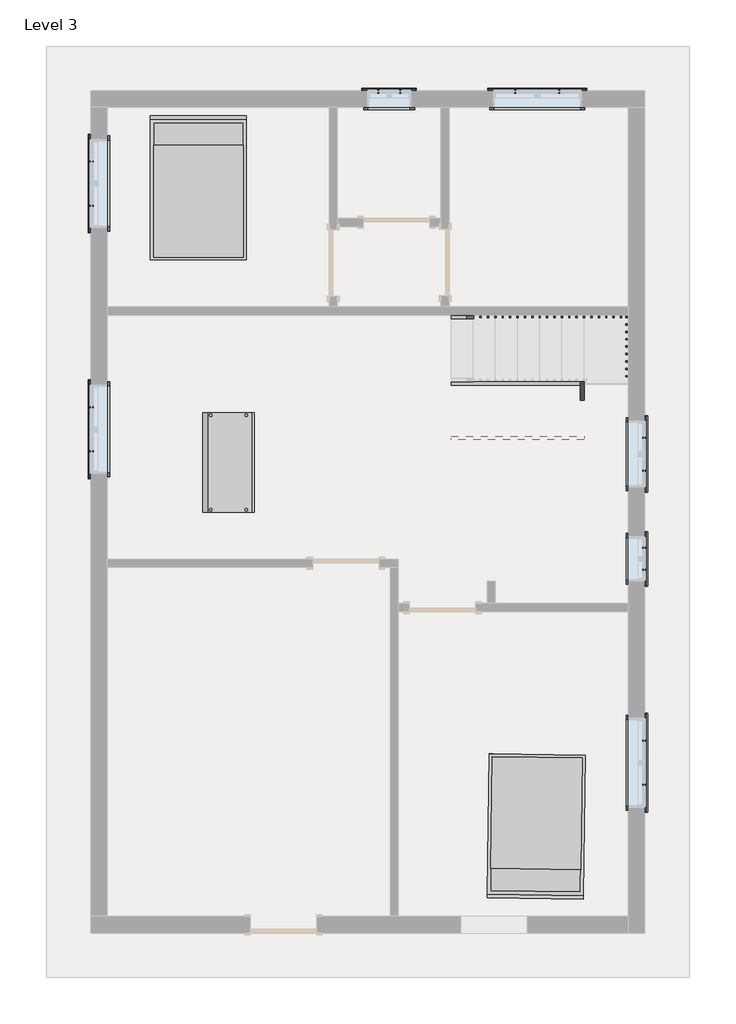
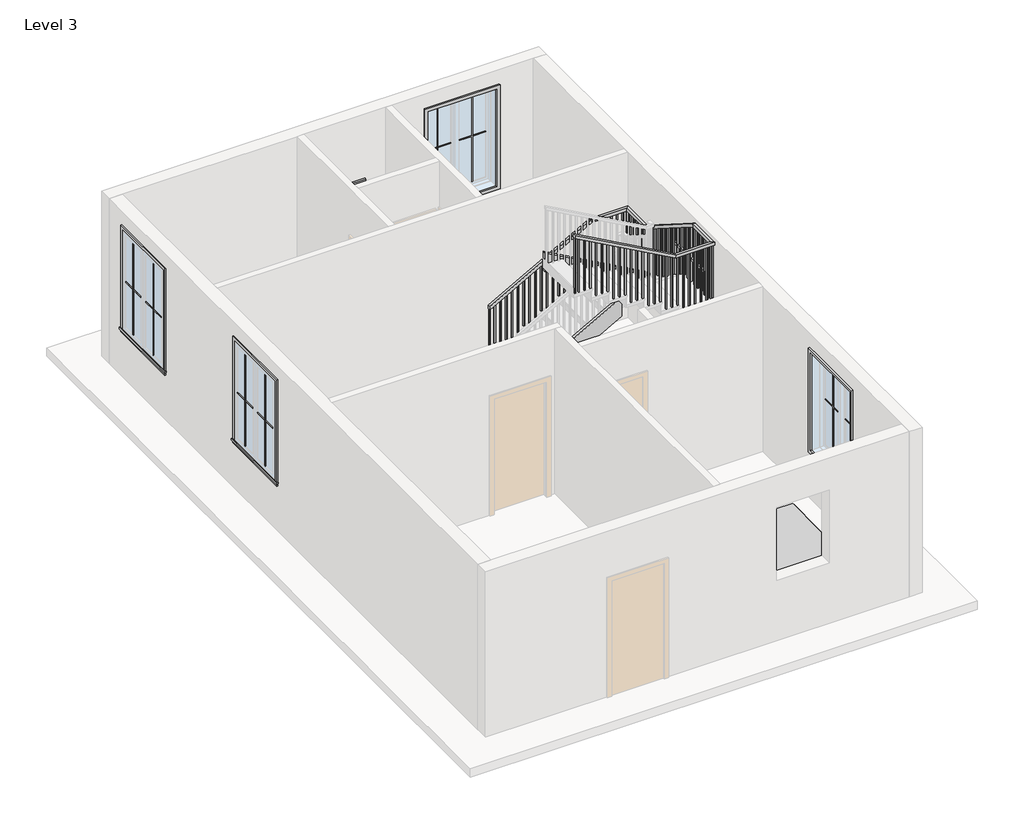
# One storey, part 2 of 2: 29 proxies, 3 members, 2 furniture elements, 1 railing.
"""IFC4 building model written with IfcOpenShell, lengths in millimetres."""

from ifc_helpers import new_model, si_unit, frame, origin, place, context, project, spatial, polyline, outline, extrude, faceted_brep, transform, mapped, element, save
from components import modern_coffee_table_17989_modern_coffee_table_17989_d3a860c8, muntin_pattern_2x2_muntin_pattern_2x2_2b4d9f72, muntin_pattern_2x2_muntin_pattern_2x2_ef995ed3, muntin_pattern_2x2_muntin_pattern_2x2_53152e2c, muntin_pattern_2x2_muntin_pattern_2x2_e8f3e573, muntin_pattern_2x2_muntin_pattern_2x2_9b64c8d5, muntin_pattern_2x2_muntin_pattern_2x2_d319fd2e, trim_window_exterior_flat_with_sill_b7e4d11c, trim_window_exterior_flat_with_sill_a665a915, trim_window_exterior_flat_with_sill_66148908, trim_window_interior_flat_picture_frame_936b8d2a, trim_window_interior_flat_picture_frame_d485c387, trim_window_interior_flat_picture_frame_d5b7f3a4, bed_17739_bed_17739_15c61121

model = new_model("IFC4")

# Units and contexts
model_context = context("Model", 3, world=origin())
ifc_project = project(units=[si_unit("LENGTHUNIT", "METRE", prefix="MILLI")], contexts=[model_context])

# Site, building, storey
site = spatial("IfcSite", under=ifc_project)
building = spatial("IfcBuilding", under=site)
storey = spatial("IfcBuildingStorey", under=building, Name="Level 3", Elevation=6096.0)

# Proxies
placement = place(None, origin())
modern_coffee_table_17989_modern_coffee_table_17989_shape = modern_coffee_table_17989_modern_coffee_table_17989_d3a860c8(model_context)
element("IfcBuildingElementProxy", 1, Name="Modern_Coffee_Table_17989 : Modern_Coffee_Table_17989", ObjectType="Modern_Coffee_Table_17989 : Modern_Coffee_Table_17989", at=placement, inside=storey, context=model_context, shape_type="MappedRepresentation", body=[
    mapped(modern_coffee_table_17989_modern_coffee_table_17989_shape, transform((3060.7, 9172.1823212, 6096.0), x_axis=(0.0, 1.0, 0.0), y_axis=(-1.0, 0.0, 0.0), z_axis=(0.0, 0.0, 1.0))),
])
muntin_pattern_2x2_muntin_pattern_2x2_shape = muntin_pattern_2x2_muntin_pattern_2x2_2b4d9f72(model_context)
element("IfcBuildingElementProxy", 2, Name="Muntin Pattern_2x2 : Muntin Pattern_2x2", ObjectType="Muntin Pattern_2x2 : Muntin Pattern_2x2", at=placement, inside=storey, context=model_context, shape_type="MappedRepresentation", body=[
    mapped(muntin_pattern_2x2_muntin_pattern_2x2_shape, transform((1533.525, 12477.4069306, 7080.25), x_axis=(0.0, 1.0, 0.0), y_axis=(-1.0, 0.0, 0.0), z_axis=(0.0, 0.0, 1.0))),
])
element("IfcBuildingElementProxy", 3, Name="Muntin Pattern_2x2 : Muntin Pattern_2x2", ObjectType="Muntin Pattern_2x2 : Muntin Pattern_2x2", at=placement, inside=storey, context=model_context, shape_type="MappedRepresentation", body=[
    mapped(muntin_pattern_2x2_muntin_pattern_2x2_shape, transform((7361.2375, 14045.8073212, 7080.25), x_axis=(1.0, 0.0, 0.0), y_axis=(0.0, 1.0, 0.0), z_axis=(0.0, 0.0, 1.0))),
])
element("IfcBuildingElementProxy", 4, Name="Muntin Pattern_2x2 : Muntin Pattern_2x2", ObjectType="Muntin Pattern_2x2 : Muntin Pattern_2x2", at=placement, inside=storey, context=model_context, shape_type="MappedRepresentation", body=[
    mapped(muntin_pattern_2x2_muntin_pattern_2x2_shape, transform((9134.475, 5119.2948212, 7080.25), x_axis=(0.0, -1.0, 0.0), y_axis=(1.0, 0.0, 0.0), z_axis=(0.0, 0.0, 1.0))),
])
element("IfcBuildingElementProxy", 5, Name="Muntin Pattern_2x2 : Muntin Pattern_2x2", ObjectType="Muntin Pattern_2x2 : Muntin Pattern_2x2", at=placement, inside=storey, context=model_context, shape_type="MappedRepresentation", body=[
    mapped(muntin_pattern_2x2_muntin_pattern_2x2_shape, transform((1533.525, 9097.5698212, 7080.25), x_axis=(0.0, 1.0, 0.0), y_axis=(-1.0, 0.0, 0.0), z_axis=(0.0, 0.0, 1.0))),
])
muntin_pattern_2x2_muntin_pattern_2x2_2_shape = muntin_pattern_2x2_muntin_pattern_2x2_ef995ed3(model_context)
element("IfcBuildingElementProxy", 6, Name="Muntin Pattern_2x2 : Muntin Pattern_2x2", ObjectType="Muntin Pattern_2x2 : Muntin Pattern_2x2", at=placement, inside=storey, context=model_context, shape_type="MappedRepresentation", body=[
    mapped(muntin_pattern_2x2_muntin_pattern_2x2_2_shape, transform((1533.525, 13083.8319306, 7080.25), x_axis=(0.0, -1.0, 0.0), y_axis=(1.0, 0.0, 0.0), z_axis=(0.0, 0.0, 1.0))),
])
element("IfcBuildingElementProxy", 7, Name="Muntin Pattern_2x2 : Muntin Pattern_2x2", ObjectType="Muntin Pattern_2x2 : Muntin Pattern_2x2", at=placement, inside=storey, context=model_context, shape_type="MappedRepresentation", body=[
    mapped(muntin_pattern_2x2_muntin_pattern_2x2_2_shape, transform((7967.6625, 14045.8073212, 7080.25), x_axis=(-1.0, 0.0, 0.0), y_axis=(0.0, -1.0, 0.0), z_axis=(0.0, 0.0, 1.0))),
])
element("IfcBuildingElementProxy", 8, Name="Muntin Pattern_2x2 : Muntin Pattern_2x2", ObjectType="Muntin Pattern_2x2 : Muntin Pattern_2x2", at=placement, inside=storey, context=model_context, shape_type="MappedRepresentation", body=[
    mapped(muntin_pattern_2x2_muntin_pattern_2x2_2_shape, transform((9134.475, 4512.8698212, 7080.25), x_axis=(0.0, 1.0, 0.0), y_axis=(-1.0, 0.0, 0.0), z_axis=(0.0, 0.0, 1.0))),
])
element("IfcBuildingElementProxy", 9, Name="Muntin Pattern_2x2 : Muntin Pattern_2x2", ObjectType="Muntin Pattern_2x2 : Muntin Pattern_2x2", at=placement, inside=storey, context=model_context, shape_type="MappedRepresentation", body=[
    mapped(muntin_pattern_2x2_muntin_pattern_2x2_2_shape, transform((1533.525, 9703.9948212, 7080.25), x_axis=(0.0, -1.0, 0.0), y_axis=(1.0, 0.0, 0.0), z_axis=(0.0, 0.0, 1.0))),
])
muntin_pattern_2x2_muntin_pattern_2x2_3_shape = muntin_pattern_2x2_muntin_pattern_2x2_53152e2c(model_context)
element("IfcBuildingElementProxy", 10, Name="Muntin Pattern_2x2 : Muntin Pattern_2x2", ObjectType="Muntin Pattern_2x2 : Muntin Pattern_2x2", at=placement, inside=storey, context=model_context, shape_type="MappedRepresentation", body=[
    mapped(muntin_pattern_2x2_muntin_pattern_2x2_3_shape, transform((9134.475, 7771.2135712, 7080.25), x_axis=(0.0, -1.0, 0.0), y_axis=(1.0, 0.0, 0.0), z_axis=(0.0, 0.0, 1.0))),
])
element("IfcBuildingElementProxy", 11, Name="Muntin Pattern_2x2 : Muntin Pattern_2x2", ObjectType="Muntin Pattern_2x2 : Muntin Pattern_2x2", at=placement, inside=storey, context=model_context, shape_type="MappedRepresentation", body=[
    mapped(muntin_pattern_2x2_muntin_pattern_2x2_3_shape, transform((5475.2875, 14045.8073212, 7080.25), x_axis=(1.0, 0.0, 0.0), y_axis=(0.0, 1.0, 0.0), z_axis=(0.0, 0.0, 1.0))),
])
muntin_pattern_2x2_muntin_pattern_2x2_4_shape = muntin_pattern_2x2_muntin_pattern_2x2_e8f3e573(model_context)
element("IfcBuildingElementProxy", 12, Name="Muntin Pattern_2x2 : Muntin Pattern_2x2", ObjectType="Muntin Pattern_2x2 : Muntin Pattern_2x2", at=placement, inside=storey, context=model_context, shape_type="MappedRepresentation", body=[
    mapped(muntin_pattern_2x2_muntin_pattern_2x2_4_shape, transform((9134.475, 7469.5885712, 7080.25), x_axis=(0.0, 1.0, 0.0), y_axis=(-1.0, 0.0, 0.0), z_axis=(0.0, 0.0, 1.0))),
])
element("IfcBuildingElementProxy", 13, Name="Muntin Pattern_2x2 : Muntin Pattern_2x2", ObjectType="Muntin Pattern_2x2 : Muntin Pattern_2x2", at=placement, inside=storey, context=model_context, shape_type="MappedRepresentation", body=[
    mapped(muntin_pattern_2x2_muntin_pattern_2x2_4_shape, transform((5776.9125, 14045.8073212, 7080.25), x_axis=(-1.0, 0.0, 0.0), y_axis=(0.0, -1.0, 0.0), z_axis=(0.0, 0.0, 1.0))),
])
muntin_pattern_2x2_muntin_pattern_2x2_5_shape = muntin_pattern_2x2_muntin_pattern_2x2_9b64c8d5(model_context)
element("IfcBuildingElementProxy", 14, Name="Muntin Pattern_2x2 : Muntin Pattern_2x2", ObjectType="Muntin Pattern_2x2 : Muntin Pattern_2x2", at=placement, inside=storey, context=model_context, shape_type="MappedRepresentation", body=[
    mapped(muntin_pattern_2x2_muntin_pattern_2x2_5_shape, transform((9134.475, 9287.1024384, 7080.25), x_axis=(0.0, -1.0, 0.0), y_axis=(1.0, 0.0, 0.0), z_axis=(0.0, 0.0, 1.0))),
])
muntin_pattern_2x2_muntin_pattern_2x2_6_shape = muntin_pattern_2x2_muntin_pattern_2x2_d319fd2e(model_context)
element("IfcBuildingElementProxy", 15, Name="Muntin Pattern_2x2 : Muntin Pattern_2x2", ObjectType="Muntin Pattern_2x2 : Muntin Pattern_2x2", at=placement, inside=storey, context=model_context, shape_type="MappedRepresentation", body=[
    mapped(muntin_pattern_2x2_muntin_pattern_2x2_6_shape, transform((9134.475, 8833.0774384, 7080.25), x_axis=(0.0, 1.0, 0.0), y_axis=(-1.0, 0.0, 0.0), z_axis=(0.0, 0.0, 1.0))),
])
trim_window_exterior_flat_with_sill_shape = trim_window_exterior_flat_with_sill_b7e4d11c(model_context)
element("IfcBuildingElementProxy", 16, Name="Trim-Window-Exterior-Flat : with Sill", ObjectType="Trim-Window-Exterior-Flat : with Sill", at=placement, inside=storey, context=model_context, shape_type="MappedRepresentation", body=[
    mapped(trim_window_exterior_flat_with_sill_shape, transform((1524.0, 12780.6194306, 8839.2), x_axis=(0.0, -1.0, 0.0), y_axis=(0.0, 0.0, 1.0), z_axis=(-1.0, 0.0, 0.0))),
])
element("IfcBuildingElementProxy", 17, Name="Trim-Window-Exterior-Flat : with Sill", ObjectType="Trim-Window-Exterior-Flat : with Sill", at=placement, inside=storey, context=model_context, shape_type="MappedRepresentation", body=[
    mapped(trim_window_exterior_flat_with_sill_shape, transform((7664.45, 14055.3323212, 8839.2), x_axis=(-1.0, 0.0, 0.0), y_axis=(0.0, 0.0, 1.0), z_axis=(0.0, 1.0, 0.0))),
])
element("IfcBuildingElementProxy", 18, Name="Trim-Window-Exterior-Flat : with Sill", ObjectType="Trim-Window-Exterior-Flat : with Sill", at=placement, inside=storey, context=model_context, shape_type="MappedRepresentation", body=[
    mapped(trim_window_exterior_flat_with_sill_shape, transform((9144.0, 4816.0823212, 8839.2), x_axis=(0.0, 1.0, 0.0), y_axis=(0.0, 0.0, 1.0), z_axis=(1.0, 0.0, 0.0))),
])
element("IfcBuildingElementProxy", 19, Name="Trim-Window-Exterior-Flat : with Sill", ObjectType="Trim-Window-Exterior-Flat : with Sill", at=placement, inside=storey, context=model_context, shape_type="MappedRepresentation", body=[
    mapped(trim_window_exterior_flat_with_sill_shape, transform((1524.0, 9400.7823212, 8839.2), x_axis=(0.0, -1.0, 0.0), y_axis=(0.0, 0.0, 1.0), z_axis=(-1.0, 0.0, 0.0))),
])
trim_window_exterior_flat_with_sill_2_shape = trim_window_exterior_flat_with_sill_a665a915(model_context)
element("IfcBuildingElementProxy", 20, Name="Trim-Window-Exterior-Flat : with Sill", ObjectType="Trim-Window-Exterior-Flat : with Sill", at=placement, inside=storey, context=model_context, shape_type="MappedRepresentation", body=[
    mapped(trim_window_exterior_flat_with_sill_2_shape, transform((9144.0, 7620.4010712, 7924.8), x_axis=(0.0, 1.0, 0.0), y_axis=(0.0, 0.0, 1.0), z_axis=(1.0, 0.0, 0.0))),
])
element("IfcBuildingElementProxy", 21, Name="Trim-Window-Exterior-Flat : with Sill", ObjectType="Trim-Window-Exterior-Flat : with Sill", at=placement, inside=storey, context=model_context, shape_type="MappedRepresentation", body=[
    mapped(trim_window_exterior_flat_with_sill_2_shape, transform((5626.1, 14055.3323212, 7924.8), x_axis=(-1.0, 0.0, 0.0), y_axis=(0.0, 0.0, 1.0), z_axis=(0.0, 1.0, 0.0))),
])
trim_window_exterior_flat_with_sill_3_shape = trim_window_exterior_flat_with_sill_66148908(model_context)
element("IfcBuildingElementProxy", 22, Name="Trim-Window-Exterior-Flat : with Sill", ObjectType="Trim-Window-Exterior-Flat : with Sill", at=placement, inside=storey, context=model_context, shape_type="MappedRepresentation", body=[
    mapped(trim_window_exterior_flat_with_sill_3_shape, transform((9144.0, 9060.0899384, 8356.6), x_axis=(0.0, 1.0, 0.0), y_axis=(0.0, 0.0, 1.0), z_axis=(1.0, 0.0, 0.0))),
])
trim_window_interior_flat_picture_frame_shape = trim_window_interior_flat_picture_frame_936b8d2a(model_context)
element("IfcBuildingElementProxy", 23, Name="Trim-Window-Interior-Flat : Picture Frame", ObjectType="Trim-Window-Interior-Flat : Picture Frame", at=placement, inside=storey, context=model_context, shape_type="MappedRepresentation", body=[
    mapped(trim_window_interior_flat_picture_frame_shape, transform((1752.6, 12780.6194306, 8839.2), x_axis=(0.0, 1.0, 0.0), y_axis=(0.0, 0.0, 1.0), z_axis=(1.0, 0.0, 0.0))),
])
element("IfcBuildingElementProxy", 24, Name="Trim-Window-Interior-Flat : Picture Frame", ObjectType="Trim-Window-Interior-Flat : Picture Frame", at=placement, inside=storey, context=model_context, shape_type="MappedRepresentation", body=[
    mapped(trim_window_interior_flat_picture_frame_shape, transform((7664.45, 13826.7323212, 8839.2), x_axis=(1.0, 0.0, 0.0), y_axis=(0.0, 0.0, 1.0), z_axis=(0.0, -1.0, 0.0))),
])
element("IfcBuildingElementProxy", 25, Name="Trim-Window-Interior-Flat : Picture Frame", ObjectType="Trim-Window-Interior-Flat : Picture Frame", at=placement, inside=storey, context=model_context, shape_type="MappedRepresentation", body=[
    mapped(trim_window_interior_flat_picture_frame_shape, transform((8915.4, 4816.0823212, 8839.2), x_axis=(0.0, -1.0, 0.0), y_axis=(0.0, 0.0, 1.0), z_axis=(-1.0, 0.0, 0.0))),
])
element("IfcBuildingElementProxy", 26, Name="Trim-Window-Interior-Flat : Picture Frame", ObjectType="Trim-Window-Interior-Flat : Picture Frame", at=placement, inside=storey, context=model_context, shape_type="MappedRepresentation", body=[
    mapped(trim_window_interior_flat_picture_frame_shape, transform((1752.6, 9400.7823212, 8839.2), x_axis=(0.0, 1.0, 0.0), y_axis=(0.0, 0.0, 1.0), z_axis=(1.0, 0.0, 0.0))),
])
trim_window_interior_flat_picture_frame_2_shape = trim_window_interior_flat_picture_frame_d485c387(model_context)
element("IfcBuildingElementProxy", 27, Name="Trim-Window-Interior-Flat : Picture Frame", ObjectType="Trim-Window-Interior-Flat : Picture Frame", at=placement, inside=storey, context=model_context, shape_type="MappedRepresentation", body=[
    mapped(trim_window_interior_flat_picture_frame_2_shape, transform((8915.4, 7620.4010712, 7924.8), x_axis=(0.0, -1.0, 0.0), y_axis=(0.0, 0.0, 1.0), z_axis=(-1.0, 0.0, 0.0))),
])
element("IfcBuildingElementProxy", 28, Name="Trim-Window-Interior-Flat : Picture Frame", ObjectType="Trim-Window-Interior-Flat : Picture Frame", at=placement, inside=storey, context=model_context, shape_type="MappedRepresentation", body=[
    mapped(trim_window_interior_flat_picture_frame_2_shape, transform((5626.1, 13826.7323212, 7924.8), x_axis=(1.0, 0.0, 0.0), y_axis=(0.0, 0.0, 1.0), z_axis=(0.0, -1.0, 0.0))),
])
trim_window_interior_flat_picture_frame_3_shape = trim_window_interior_flat_picture_frame_d5b7f3a4(model_context)
element("IfcBuildingElementProxy", 29, Name="Trim-Window-Interior-Flat : Picture Frame", ObjectType="Trim-Window-Interior-Flat : Picture Frame", at=placement, inside=storey, context=model_context, shape_type="MappedRepresentation", body=[
    mapped(trim_window_interior_flat_picture_frame_3_shape, transform((8915.4, 9060.0899384, 8356.6), x_axis=(0.0, -1.0, 0.0), y_axis=(0.0, 0.0, 1.0), z_axis=(-1.0, 0.0, 0.0))),
])

# Furniture
bed_17739_bed_17739_shape = bed_17739_bed_17739_15c61121(model_context)
element("IfcFurniture", 30, ObjectType="Bed_17739 : Bed_17739", at=placement, inside=storey, context=model_context, shape_type="MappedRepresentation", body=[
    mapped(bed_17739_bed_17739_shape, transform((3003.55, 12696.4323212, 6096.0), x_axis=(1.0, 0.0, 0.0), y_axis=(0.0, 1.0, 0.0), z_axis=(0.0, 0.0, 1.0))),
])
element("IfcFurniture", 31, ObjectType="Bed_17739 : Bed_17739", at=placement, inside=storey, context=model_context, shape_type="MappedRepresentation", body=[
    mapped(bed_17739_bed_17739_shape, transform((7650.1504891, 3963.5673274, 6096.0), x_axis=(-0.9999063358908578, 0.013686469424921632, 0.0), y_axis=(-0.013686469424921632, -0.9999063358908578, 0.0), z_axis=(0.0, 0.0, 1.0))),
])

# Members
element("IfcMember", 32, ObjectType="Stringer - 2\" Width", at=placement, inside=storey, context=model_context, shape_type="SweptSolid", body=[
    extrude(outline(polyline([(6303.5983948, 6477.0), (6096.0, 6477.0), (6096.0, 6730.9445028), (6942.6974984, 8255.0), (7291.3761726, 8255.0), (6303.5983948, 6477.0)])), frame((0.0, 10004.0323212, 0.0), z_axis=(0.0, 1.0, 0.0), x_axis=(0.0, 0.0, 1.0)), (0.0, 0.0, 1.0), 50.8),
])
element("IfcMember", 33, ObjectType="Stringer - 2\" Width", at=placement, inside=storey, context=model_context, shape_type="SweptSolid", body=[
    extrude(outline(polyline([(10054.8323212, 7496.2030053), (10054.8323212, 7135.1566026), (9305.5323212, 7610.9026344), (9305.5323212, 7971.949037), (10054.8323212, 7496.2030053)])), frame((8255.0, 0.0, 0.0), z_axis=(1.0, 0.0, 0.0), x_axis=(0.0, 1.0, 0.0)), (0.0, 0.0, 1.0), 50.8),
])
element("IfcMember", 34, ObjectType="Stringer - 2\" Width", at=placement, inside=storey, context=model_context, shape_type="SweptSolid", body=[
    extrude(outline(polyline([(7817.5863873, 8305.8), (8166.2650614, 8305.8), (9182.2650614, 6477.0), (8833.5863873, 6477.0), (7817.5863873, 8305.8)])), frame((0.0, 9254.7323212, 0.0), z_axis=(0.0, 1.0, 0.0), x_axis=(0.0, 0.0, 1.0)), (0.0, 0.0, 1.0), 50.8),
])

# Railing
element("IfcRailing", 35, ObjectType="Handrail - Rectangular", at=placement, inside=storey, context=model_context, shape_type="SolidModel", body=[
    faceted_brep([(6477.0, 10969.2323212, 7179.7333333), (6477.0, 10969.2323212, 7121.620221), (6477.0, 10918.4323212, 7121.620221), (6477.0, 10918.4323212, 7179.7333333), (8242.3, 10969.2323212, 8160.4555556), (8255.4636022, 10969.2323212, 8109.6555556), (8255.4636022, 10918.4323212, 8109.6555556), (8242.3, 10918.4323212, 8160.4555556), (8915.4, 10969.2323212, 8160.4555556), (8915.4, 10969.2323212, 8109.6555556), (8864.6, 10918.4323212, 8109.6555556), (8864.6, 10918.4323212, 8160.4555556), (8915.4, 10377.0948212, 8160.4555556), (8915.4, 10362.3301405, 8109.6555556), (8864.6, 10362.3301405, 8109.6555556), (8864.6, 10377.0948212, 8160.4555556), (8915.4, 8932.4698212, 9077.6777778), (8915.4, 8917.7051405, 9026.8777778), (8864.6, 8917.7051405, 9026.8777778), (8864.6, 8932.4698212, 9077.6777778), (8915.4, 8340.3323212, 9077.6777778), (8915.4, 8340.3323212, 9026.8777778), (8864.6, 8391.1323212, 9026.8777778), (8864.6, 8391.1323212, 9077.6777778), (8242.3, 8340.3323212, 9077.6777778), (8229.1363978, 8340.3323212, 9026.8777778), (8229.1363978, 8391.1323212, 9026.8777778), (8242.3, 8391.1323212, 9077.6777778), (6477.0, 8340.3323212, 10058.4), (6477.0, 8391.1323212, 10058.4), (6477.0, 8391.1323212, 10000.2868876), (6477.0, 8340.3323212, 10000.2868876)], [[[0, 1, 2, 3]], [[1, 0, 4, 5]], [[2, 1, 5, 6]], [[3, 2, 6, 7]], [[0, 3, 7, 4]], [[5, 4, 8, 9]], [[6, 5, 9, 10]], [[7, 6, 10, 11]], [[4, 7, 11, 8]], [[9, 8, 12, 13]], [[10, 9, 13, 14]], [[11, 10, 14, 15]], [[8, 11, 15, 12]], [[13, 12, 16, 17]], [[14, 13, 17, 18]], [[15, 14, 18, 19]], [[12, 15, 19, 16]], [[17, 16, 20, 21]], [[18, 17, 21, 22]], [[19, 18, 22, 23]], [[16, 19, 23, 20]], [[21, 20, 24, 25]], [[22, 21, 25, 26]], [[23, 22, 26, 27]], [[20, 23, 27, 24]], [[28, 29, 30, 31]], [[25, 24, 28, 31]], [[26, 25, 31, 30]], [[27, 26, 30, 29]], [[24, 27, 29, 28]]]),
    extrude(outline(polyline([(9963.245221, 6543.675), (8974.6666667, 6543.675), (8974.6666667, 6562.725), (9952.6618876, 6562.725), (9963.245221, 6543.675)])), frame((0.0, 8356.2073212, 0.0), z_axis=(0.0, 1.0, 0.0), x_axis=(0.0, 0.0, 1.0)), (0.0, 0.0, 1.0), 19.05),
    extrude(outline(polyline([(9906.8007765, 6645.275), (8974.6666667, 6645.275), (8974.6666667, 6664.325), (9896.2174432, 6664.325), (9906.8007765, 6645.275)])), frame((0.0, 8356.2073212, 0.0), z_axis=(0.0, 1.0, 0.0), x_axis=(0.0, 0.0, 1.0)), (0.0, 0.0, 1.0), 19.05),
    extrude(outline(polyline([(9850.3563321, 6746.875), (8974.6666667, 6746.875), (8974.6666667, 6765.925), (9839.7729988, 6765.925), (9850.3563321, 6746.875)])), frame((0.0, 8356.2073212, 0.0), z_axis=(0.0, 1.0, 0.0), x_axis=(0.0, 0.0, 1.0)), (0.0, 0.0, 1.0), 19.05),
    extrude(outline(polyline([(9793.9118876, 6848.475), (8805.3333333, 6848.475), (8805.3333333, 6867.525), (9783.3285543, 6867.525), (9793.9118876, 6848.475)])), frame((0.0, 8356.2073212, 0.0), z_axis=(0.0, 1.0, 0.0), x_axis=(0.0, 0.0, 1.0)), (0.0, 0.0, 1.0), 19.05),
    extrude(outline(polyline([(9737.4674432, 6950.075), (8805.3333333, 6950.075), (8805.3333333, 6969.125), (9726.8841099, 6969.125), (9737.4674432, 6950.075)])), frame((0.0, 8356.2073212, 0.0), z_axis=(0.0, 1.0, 0.0), x_axis=(0.0, 0.0, 1.0)), (0.0, 0.0, 1.0), 19.05),
    extrude(outline(polyline([(9681.0229988, 7051.675), (8805.3333333, 7051.675), (8805.3333333, 7070.725), (9670.4396654, 7070.725), (9681.0229988, 7051.675)])), frame((0.0, 8356.2073212, 0.0), z_axis=(0.0, 1.0, 0.0), x_axis=(0.0, 0.0, 1.0)), (0.0, 0.0, 1.0), 19.05),
    extrude(outline(polyline([(9624.5785543, 7153.275), (8636.0, 7153.275), (8636.0, 7172.325), (9613.995221, 7172.325), (9624.5785543, 7153.275)])), frame((0.0, 8356.2073212, 0.0), z_axis=(0.0, 1.0, 0.0), x_axis=(0.0, 0.0, 1.0)), (0.0, 0.0, 1.0), 19.05),
    extrude(outline(polyline([(9568.1341099, 7254.875), (8636.0, 7254.875), (8636.0, 7273.925), (9557.5507765, 7273.925), (9568.1341099, 7254.875)])), frame((0.0, 8356.2073212, 0.0), z_axis=(0.0, 1.0, 0.0), x_axis=(0.0, 0.0, 1.0)), (0.0, 0.0, 1.0), 19.05),
    extrude(outline(polyline([(9511.6896654, 7356.475), (8636.0, 7356.475), (8636.0, 7375.525), (9501.1063321, 7375.525), (9511.6896654, 7356.475)])), frame((0.0, 8356.2073212, 0.0), z_axis=(0.0, 1.0, 0.0), x_axis=(0.0, 0.0, 1.0)), (0.0, 0.0, 1.0), 19.05),
    extrude(outline(polyline([(9455.245221, 7458.075), (8466.6666667, 7458.075), (8466.6666667, 7477.125), (9444.6618876, 7477.125), (9455.245221, 7458.075)])), frame((0.0, 8356.2073212, 0.0), z_axis=(0.0, 1.0, 0.0), x_axis=(0.0, 0.0, 1.0)), (0.0, 0.0, 1.0), 19.05),
    extrude(outline(polyline([(9398.8007765, 7559.675), (8466.6666667, 7559.675), (8466.6666667, 7578.725), (9388.2174432, 7578.725), (9398.8007765, 7559.675)])), frame((0.0, 8356.2073212, 0.0), z_axis=(0.0, 1.0, 0.0), x_axis=(0.0, 0.0, 1.0)), (0.0, 0.0, 1.0), 19.05),
    extrude(outline(polyline([(9342.3563321, 7661.275), (8466.6666667, 7661.275), (8466.6666667, 7680.325), (9331.7729988, 7680.325), (9342.3563321, 7661.275)])), frame((0.0, 8356.2073212, 0.0), z_axis=(0.0, 1.0, 0.0), x_axis=(0.0, 0.0, 1.0)), (0.0, 0.0, 1.0), 19.05),
    extrude(outline(polyline([(9285.9118876, 7762.875), (8297.3333333, 7762.875), (8297.3333333, 7781.925), (9275.3285543, 7781.925), (9285.9118876, 7762.875)])), frame((0.0, 8356.2073212, 0.0), z_axis=(0.0, 1.0, 0.0), x_axis=(0.0, 0.0, 1.0)), (0.0, 0.0, 1.0), 19.05),
    extrude(outline(polyline([(9229.4674432, 7864.475), (8297.3333333, 7864.475), (8297.3333333, 7883.525), (9218.8841099, 7883.525), (9229.4674432, 7864.475)])), frame((0.0, 8356.2073212, 0.0), z_axis=(0.0, 1.0, 0.0), x_axis=(0.0, 0.0, 1.0)), (0.0, 0.0, 1.0), 19.05),
    extrude(outline(polyline([(9173.0229988, 7966.075), (8297.3333333, 7966.075), (8297.3333333, 7985.125), (9162.4396654, 7985.125), (9173.0229988, 7966.075)])), frame((0.0, 8356.2073212, 0.0), z_axis=(0.0, 1.0, 0.0), x_axis=(0.0, 0.0, 1.0)), (0.0, 0.0, 1.0), 19.05),
    extrude(outline(polyline([(9116.5785543, 8067.675), (8128.0, 8067.675), (8128.0, 8086.725), (9105.995221, 8086.725), (9116.5785543, 8067.675)])), frame((0.0, 8356.2073212, 0.0), z_axis=(0.0, 1.0, 0.0), x_axis=(0.0, 0.0, 1.0)), (0.0, 0.0, 1.0), 19.05),
    extrude(outline(polyline([(9060.1341099, 8169.275), (8128.0, 8169.275), (8128.0, 8188.325), (9049.5507765, 8188.325), (9060.1341099, 8169.275)])), frame((0.0, 8356.2073212, 0.0), z_axis=(0.0, 1.0, 0.0), x_axis=(0.0, 0.0, 1.0)), (0.0, 0.0, 1.0), 19.05),
    extrude(outline(polyline([(8289.925, 8356.2073212), (8270.875, 8356.2073212), (8270.875, 8375.2573212), (8289.925, 8375.2573212), (8289.925, 8356.2073212)])), frame((0.0, 0.0, 8128.0), z_axis=(0.0, 0.0, 1.0), x_axis=(1.0, 0.0, 0.0)), (0.0, 0.0, 1.0), 898.8777778),
    extrude(outline(polyline([(8391.525, 8356.2073212), (8372.475, 8356.2073212), (8372.475, 8375.2573212), (8391.525, 8375.2573212), (8391.525, 8356.2073212)])), frame((0.0, 0.0, 7958.6666667), z_axis=(0.0, 0.0, 1.0), x_axis=(1.0, 0.0, 0.0)), (0.0, 0.0, 1.0), 1068.2111111),
    extrude(outline(polyline([(8493.125, 8356.2073212), (8474.075, 8356.2073212), (8474.075, 8375.2573212), (8493.125, 8375.2573212), (8493.125, 8356.2073212)])), frame((0.0, 0.0, 7958.6666667), z_axis=(0.0, 0.0, 1.0), x_axis=(1.0, 0.0, 0.0)), (0.0, 0.0, 1.0), 1068.2111111),
    extrude(outline(polyline([(8594.725, 8356.2073212), (8575.675, 8356.2073212), (8575.675, 8375.2573212), (8594.725, 8375.2573212), (8594.725, 8356.2073212)])), frame((0.0, 0.0, 7958.6666667), z_axis=(0.0, 0.0, 1.0), x_axis=(1.0, 0.0, 0.0)), (0.0, 0.0, 1.0), 1068.2111111),
    extrude(outline(polyline([(8696.325, 8356.2073212), (8677.275, 8356.2073212), (8677.275, 8375.2573212), (8696.325, 8375.2573212), (8696.325, 8356.2073212)])), frame((0.0, 0.0, 7958.6666667), z_axis=(0.0, 0.0, 1.0), x_axis=(1.0, 0.0, 0.0)), (0.0, 0.0, 1.0), 1068.2111111),
    extrude(outline(polyline([(8797.925, 8356.2073212), (8778.875, 8356.2073212), (8778.875, 8375.2573212), (8797.925, 8375.2573212), (8797.925, 8356.2073212)])), frame((0.0, 0.0, 7958.6666667), z_axis=(0.0, 0.0, 1.0), x_axis=(1.0, 0.0, 0.0)), (0.0, 0.0, 1.0), 1068.2111111),
    extrude(outline(polyline([(8899.525, 8413.3573212), (8899.525, 8394.3073212), (8880.475, 8394.3073212), (8880.475, 8413.3573212), (8899.525, 8413.3573212)])), frame((0.0, 0.0, 7958.6666667), z_axis=(0.0, 0.0, 1.0), x_axis=(1.0, 0.0, 0.0)), (0.0, 0.0, 1.0), 1068.2111111),
    extrude(outline(polyline([(8899.525, 8514.9573212), (8899.525, 8495.9073212), (8880.475, 8495.9073212), (8880.475, 8514.9573212), (8899.525, 8514.9573212)])), frame((0.0, 0.0, 7958.6666667), z_axis=(0.0, 0.0, 1.0), x_axis=(1.0, 0.0, 0.0)), (0.0, 0.0, 1.0), 1068.2111111),
    extrude(outline(polyline([(8899.525, 8616.5573212), (8899.525, 8597.5073212), (8880.475, 8597.5073212), (8880.475, 8616.5573212), (8899.525, 8616.5573212)])), frame((0.0, 0.0, 7958.6666667), z_axis=(0.0, 0.0, 1.0), x_axis=(1.0, 0.0, 0.0)), (0.0, 0.0, 1.0), 1068.2111111),
    extrude(outline(polyline([(8899.525, 8718.1573212), (8899.525, 8699.1073212), (8880.475, 8699.1073212), (8880.475, 8718.1573212), (8899.525, 8718.1573212)])), frame((0.0, 0.0, 7958.6666667), z_axis=(0.0, 0.0, 1.0), x_axis=(1.0, 0.0, 0.0)), (0.0, 0.0, 1.0), 1068.2111111),
    extrude(outline(polyline([(8899.525, 8819.7573212), (8899.525, 8800.7073212), (8880.475, 8800.7073212), (8880.475, 8819.7573212), (8899.525, 8819.7573212)])), frame((0.0, 0.0, 7958.6666667), z_axis=(0.0, 0.0, 1.0), x_axis=(1.0, 0.0, 0.0)), (0.0, 0.0, 1.0), 1068.2111111),
    extrude(outline(polyline([(8899.525, 8921.3573212), (8899.525, 8902.3073212), (8880.475, 8902.3073212), (8880.475, 8921.3573212), (8899.525, 8921.3573212)])), frame((0.0, 0.0, 7958.6666667), z_axis=(0.0, 0.0, 1.0), x_axis=(1.0, 0.0, 0.0)), (0.0, 0.0, 1.0), 1068.2111111),
    extrude(outline(polyline([(9022.9573212, 8960.0509964), (9022.9573212, 7958.6666667), (9003.9073212, 7958.6666667), (9003.9073212, 8972.1462345), (9022.9573212, 8960.0509964)])), frame((8880.475, 0.0, 0.0), z_axis=(1.0, 0.0, 0.0), x_axis=(0.0, 1.0, 0.0)), (0.0, 0.0, 1.0), 19.05),
    extrude(outline(polyline([(9124.5573212, 8895.5430599), (9124.5573212, 7958.6666667), (9105.5073212, 7958.6666667), (9105.5073212, 8907.638298), (9124.5573212, 8895.5430599)])), frame((8880.475, 0.0, 0.0), z_axis=(1.0, 0.0, 0.0), x_axis=(0.0, 1.0, 0.0)), (0.0, 0.0, 1.0), 19.05),
    extrude(outline(polyline([(9226.1573212, 8831.0351234), (9226.1573212, 7958.6666667), (9207.1073212, 7958.6666667), (9207.1073212, 8843.1303615), (9226.1573212, 8831.0351234)])), frame((8880.475, 0.0, 0.0), z_axis=(1.0, 0.0, 0.0), x_axis=(0.0, 1.0, 0.0)), (0.0, 0.0, 1.0), 19.05),
    extrude(outline(polyline([(9327.7573212, 8766.5271869), (9327.7573212, 7789.3333333), (9308.7073212, 7789.3333333), (9308.7073212, 8778.622425), (9327.7573212, 8766.5271869)])), frame((8880.475, 0.0, 0.0), z_axis=(1.0, 0.0, 0.0), x_axis=(0.0, 1.0, 0.0)), (0.0, 0.0, 1.0), 19.05),
    extrude(outline(polyline([(9429.3573212, 8702.0192504), (9429.3573212, 7789.3333333), (9410.3073212, 7789.3333333), (9410.3073212, 8714.1144884), (9429.3573212, 8702.0192504)])), frame((8880.475, 0.0, 0.0), z_axis=(1.0, 0.0, 0.0), x_axis=(0.0, 1.0, 0.0)), (0.0, 0.0, 1.0), 19.05),
    extrude(outline(polyline([(9530.9573212, 8637.5113138), (9530.9573212, 7620.0), (9511.9073212, 7620.0), (9511.9073212, 8649.6065519), (9530.9573212, 8637.5113138)])), frame((8880.475, 0.0, 0.0), z_axis=(1.0, 0.0, 0.0), x_axis=(0.0, 1.0, 0.0)), (0.0, 0.0, 1.0), 19.05),
    extrude(outline(polyline([(9632.5573212, 8573.0033773), (9632.5573212, 7620.0), (9613.5073212, 7620.0), (9613.5073212, 8585.0986154), (9632.5573212, 8573.0033773)])), frame((8880.475, 0.0, 0.0), z_axis=(1.0, 0.0, 0.0), x_axis=(0.0, 1.0, 0.0)), (0.0, 0.0, 1.0), 19.05),
    extrude(outline(polyline([(9734.1573212, 8508.4954408), (9734.1573212, 7620.0), (9715.1073212, 7620.0), (9715.1073212, 8520.5906789), (9734.1573212, 8508.4954408)])), frame((8880.475, 0.0, 0.0), z_axis=(1.0, 0.0, 0.0), x_axis=(0.0, 1.0, 0.0)), (0.0, 0.0, 1.0), 19.05),
    extrude(outline(polyline([(9835.7573212, 8443.9875043), (9835.7573212, 7450.6666667), (9816.7073212, 7450.6666667), (9816.7073212, 8456.0827424), (9835.7573212, 8443.9875043)])), frame((8880.475, 0.0, 0.0), z_axis=(1.0, 0.0, 0.0), x_axis=(0.0, 1.0, 0.0)), (0.0, 0.0, 1.0), 19.05),
    extrude(outline(polyline([(9937.3573212, 8379.4795678), (9937.3573212, 7450.6666667), (9918.3073212, 7450.6666667), (9918.3073212, 8391.5748059), (9937.3573212, 8379.4795678)])), frame((8880.475, 0.0, 0.0), z_axis=(1.0, 0.0, 0.0), x_axis=(0.0, 1.0, 0.0)), (0.0, 0.0, 1.0), 19.05),
    extrude(outline(polyline([(10038.9573212, 8314.9716313), (10038.9573212, 7450.6666667), (10019.9073212, 7450.6666667), (10019.9073212, 8327.0668694), (10038.9573212, 8314.9716313)])), frame((8880.475, 0.0, 0.0), z_axis=(1.0, 0.0, 0.0), x_axis=(0.0, 1.0, 0.0)), (0.0, 0.0, 1.0), 19.05),
    extrude(outline(polyline([(10140.5573212, 8250.4636948), (10140.5573212, 7281.3333333), (10121.5073212, 7281.3333333), (10121.5073212, 8262.5589329), (10140.5573212, 8250.4636948)])), frame((8880.475, 0.0, 0.0), z_axis=(1.0, 0.0, 0.0), x_axis=(0.0, 1.0, 0.0)), (0.0, 0.0, 1.0), 19.05),
    extrude(outline(polyline([(10242.1573212, 8185.9557583), (10242.1573212, 7281.3333333), (10223.1073212, 7281.3333333), (10223.1073212, 8198.0509964), (10242.1573212, 8185.9557583)])), frame((8880.475, 0.0, 0.0), z_axis=(1.0, 0.0, 0.0), x_axis=(0.0, 1.0, 0.0)), (0.0, 0.0, 1.0), 19.05),
    extrude(outline(polyline([(10343.7573212, 8121.4478218), (10343.7573212, 7281.3333333), (10324.7073212, 7281.3333333), (10324.7073212, 8133.5430599), (10343.7573212, 8121.4478218)])), frame((8880.475, 0.0, 0.0), z_axis=(1.0, 0.0, 0.0), x_axis=(0.0, 1.0, 0.0)), (0.0, 0.0, 1.0), 19.05),
    extrude(outline(polyline([(8899.525, 10445.3573212), (8899.525, 10426.3073212), (8880.475, 10426.3073212), (8880.475, 10445.3573212), (8899.525, 10445.3573212)])), frame((0.0, 0.0, 7281.3333333), z_axis=(0.0, 0.0, 1.0), x_axis=(1.0, 0.0, 0.0)), (0.0, 0.0, 1.0), 828.3222222),
    extrude(outline(polyline([(8899.525, 10546.9573212), (8899.525, 10527.9073212), (8880.475, 10527.9073212), (8880.475, 10546.9573212), (8899.525, 10546.9573212)])), frame((0.0, 0.0, 7281.3333333), z_axis=(0.0, 0.0, 1.0), x_axis=(1.0, 0.0, 0.0)), (0.0, 0.0, 1.0), 828.3222222),
    extrude(outline(polyline([(8899.525, 10648.5573212), (8899.525, 10629.5073212), (8880.475, 10629.5073212), (8880.475, 10648.5573212), (8899.525, 10648.5573212)])), frame((0.0, 0.0, 7281.3333333), z_axis=(0.0, 0.0, 1.0), x_axis=(1.0, 0.0, 0.0)), (0.0, 0.0, 1.0), 828.3222222),
    extrude(outline(polyline([(8899.525, 10750.1573212), (8899.525, 10731.1073212), (8880.475, 10731.1073212), (8880.475, 10750.1573212), (8899.525, 10750.1573212)])), frame((0.0, 0.0, 7281.3333333), z_axis=(0.0, 0.0, 1.0), x_axis=(1.0, 0.0, 0.0)), (0.0, 0.0, 1.0), 828.3222222),
    extrude(outline(polyline([(8899.525, 10851.7573212), (8899.525, 10832.7073212), (8880.475, 10832.7073212), (8880.475, 10851.7573212), (8899.525, 10851.7573212)])), frame((0.0, 0.0, 7281.3333333), z_axis=(0.0, 0.0, 1.0), x_axis=(1.0, 0.0, 0.0)), (0.0, 0.0, 1.0), 828.3222222),
    extrude(outline(polyline([(8804.275, 10953.3573212), (8823.325, 10953.3573212), (8823.325, 10934.3073212), (8804.275, 10934.3073212), (8804.275, 10953.3573212)])), frame((0.0, 0.0, 7281.3333333), z_axis=(0.0, 0.0, 1.0), x_axis=(1.0, 0.0, 0.0)), (0.0, 0.0, 1.0), 828.3222222),
    extrude(outline(polyline([(8702.675, 10953.3573212), (8721.725, 10953.3573212), (8721.725, 10934.3073212), (8702.675, 10934.3073212), (8702.675, 10953.3573212)])), frame((0.0, 0.0, 7281.3333333), z_axis=(0.0, 0.0, 1.0), x_axis=(1.0, 0.0, 0.0)), (0.0, 0.0, 1.0), 828.3222222),
    extrude(outline(polyline([(8601.075, 10953.3573212), (8620.125, 10953.3573212), (8620.125, 10934.3073212), (8601.075, 10934.3073212), (8601.075, 10953.3573212)])), frame((0.0, 0.0, 7281.3333333), z_axis=(0.0, 0.0, 1.0), x_axis=(1.0, 0.0, 0.0)), (0.0, 0.0, 1.0), 828.3222222),
    extrude(outline(polyline([(8499.475, 10953.3573212), (8518.525, 10953.3573212), (8518.525, 10934.3073212), (8499.475, 10934.3073212), (8499.475, 10953.3573212)])), frame((0.0, 0.0, 7281.3333333), z_axis=(0.0, 0.0, 1.0), x_axis=(1.0, 0.0, 0.0)), (0.0, 0.0, 1.0), 828.3222222),
    extrude(outline(polyline([(8397.875, 10953.3573212), (8416.925, 10953.3573212), (8416.925, 10934.3073212), (8397.875, 10934.3073212), (8397.875, 10953.3573212)])), frame((0.0, 0.0, 7281.3333333), z_axis=(0.0, 0.0, 1.0), x_axis=(1.0, 0.0, 0.0)), (0.0, 0.0, 1.0), 828.3222222),
    extrude(outline(polyline([(8296.275, 10953.3573212), (8315.325, 10953.3573212), (8315.325, 10934.3073212), (8296.275, 10934.3073212), (8296.275, 10953.3573212)])), frame((0.0, 0.0, 7281.3333333), z_axis=(0.0, 0.0, 1.0), x_axis=(1.0, 0.0, 0.0)), (0.0, 0.0, 1.0), 828.3222222),
    extrude(outline(polyline([(8075.8841099, 8194.675), (7112.0, 8194.675), (7112.0, 8213.725), (8086.4674432, 8213.725), (8075.8841099, 8194.675)])), frame((0.0, 10934.3073212, 0.0), z_axis=(0.0, 1.0, 0.0), x_axis=(0.0, 0.0, 1.0)), (0.0, 0.0, 1.0), 19.05),
    extrude(outline(polyline([(8019.4396654, 8093.075), (7112.0, 8093.075), (7112.0, 8112.125), (8030.0229988, 8112.125), (8019.4396654, 8093.075)])), frame((0.0, 10934.3073212, 0.0), z_axis=(0.0, 1.0, 0.0), x_axis=(0.0, 0.0, 1.0)), (0.0, 0.0, 1.0), 19.05),
    extrude(outline(polyline([(7962.995221, 7991.475), (7112.0, 7991.475), (7112.0, 8010.525), (7973.5785543, 8010.525), (7962.995221, 7991.475)])), frame((0.0, 10934.3073212, 0.0), z_axis=(0.0, 1.0, 0.0), x_axis=(0.0, 0.0, 1.0)), (0.0, 0.0, 1.0), 19.05),
    extrude(outline(polyline([(7906.5507765, 7889.875), (6942.6666667, 7889.875), (6942.6666667, 7908.925), (7917.1341099, 7908.925), (7906.5507765, 7889.875)])), frame((0.0, 10934.3073212, 0.0), z_axis=(0.0, 1.0, 0.0), x_axis=(0.0, 0.0, 1.0)), (0.0, 0.0, 1.0), 19.05),
    extrude(outline(polyline([(7850.1063321, 7788.275), (6942.6666667, 7788.275), (6942.6666667, 7807.325), (7860.6896654, 7807.325), (7850.1063321, 7788.275)])), frame((0.0, 10934.3073212, 0.0), z_axis=(0.0, 1.0, 0.0), x_axis=(0.0, 0.0, 1.0)), (0.0, 0.0, 1.0), 19.05),
    extrude(outline(polyline([(7793.6618876, 7686.675), (6942.6666667, 7686.675), (6942.6666667, 7705.725), (7804.245221, 7705.725), (7793.6618876, 7686.675)])), frame((0.0, 10934.3073212, 0.0), z_axis=(0.0, 1.0, 0.0), x_axis=(0.0, 0.0, 1.0)), (0.0, 0.0, 1.0), 19.05),
    extrude(outline(polyline([(7737.2174432, 7585.075), (6773.3333333, 7585.075), (6773.3333333, 7604.125), (7747.8007765, 7604.125), (7737.2174432, 7585.075)])), frame((0.0, 10934.3073212, 0.0), z_axis=(0.0, 1.0, 0.0), x_axis=(0.0, 0.0, 1.0)), (0.0, 0.0, 1.0), 19.05),
    extrude(outline(polyline([(7680.7729988, 7483.475), (6773.3333333, 7483.475), (6773.3333333, 7502.525), (7691.3563321, 7502.525), (7680.7729988, 7483.475)])), frame((0.0, 10934.3073212, 0.0), z_axis=(0.0, 1.0, 0.0), x_axis=(0.0, 0.0, 1.0)), (0.0, 0.0, 1.0), 19.05),
    extrude(outline(polyline([(7624.3285543, 7381.875), (6773.3333333, 7381.875), (6773.3333333, 7400.925), (7634.9118876, 7400.925), (7624.3285543, 7381.875)])), frame((0.0, 10934.3073212, 0.0), z_axis=(0.0, 1.0, 0.0), x_axis=(0.0, 0.0, 1.0)), (0.0, 0.0, 1.0), 19.05),
    extrude(outline(polyline([(7567.8841099, 7280.275), (6604.0, 7280.275), (6604.0, 7299.325), (7578.4674432, 7299.325), (7567.8841099, 7280.275)])), frame((0.0, 10934.3073212, 0.0), z_axis=(0.0, 1.0, 0.0), x_axis=(0.0, 0.0, 1.0)), (0.0, 0.0, 1.0), 19.05),
    extrude(outline(polyline([(7511.4396654, 7178.675), (6604.0, 7178.675), (6604.0, 7197.725), (7522.0229988, 7197.725), (7511.4396654, 7178.675)])), frame((0.0, 10934.3073212, 0.0), z_axis=(0.0, 1.0, 0.0), x_axis=(0.0, 0.0, 1.0)), (0.0, 0.0, 1.0), 19.05),
    extrude(outline(polyline([(7454.995221, 7077.075), (6604.0, 7077.075), (6604.0, 7096.125), (7465.5785543, 7096.125), (7454.995221, 7077.075)])), frame((0.0, 10934.3073212, 0.0), z_axis=(0.0, 1.0, 0.0), x_axis=(0.0, 0.0, 1.0)), (0.0, 0.0, 1.0), 19.05),
    extrude(outline(polyline([(7398.5507765, 6975.475), (6434.6666667, 6975.475), (6434.6666667, 6994.525), (7409.1341099, 6994.525), (7398.5507765, 6975.475)])), frame((0.0, 10934.3073212, 0.0), z_axis=(0.0, 1.0, 0.0), x_axis=(0.0, 0.0, 1.0)), (0.0, 0.0, 1.0), 19.05),
    extrude(outline(polyline([(7342.1063321, 6873.875), (6434.6666667, 6873.875), (6434.6666667, 6892.925), (7352.6896654, 6892.925), (7342.1063321, 6873.875)])), frame((0.0, 10934.3073212, 0.0), z_axis=(0.0, 1.0, 0.0), x_axis=(0.0, 0.0, 1.0)), (0.0, 0.0, 1.0), 19.05),
    extrude(outline(polyline([(7285.6618876, 6772.275), (6434.6666667, 6772.275), (6434.6666667, 6791.325), (7296.245221, 6791.325), (7285.6618876, 6772.275)])), frame((0.0, 10934.3073212, 0.0), z_axis=(0.0, 1.0, 0.0), x_axis=(0.0, 0.0, 1.0)), (0.0, 0.0, 1.0), 19.05),
    extrude(outline(polyline([(7229.2174432, 6670.675), (6265.3333333, 6670.675), (6265.3333333, 6689.725), (7239.8007765, 6689.725), (7229.2174432, 6670.675)])), frame((0.0, 10934.3073212, 0.0), z_axis=(0.0, 1.0, 0.0), x_axis=(0.0, 0.0, 1.0)), (0.0, 0.0, 1.0), 19.05),
    extrude(outline(polyline([(7172.7729988, 6569.075), (6265.3333333, 6569.075), (6265.3333333, 6588.125), (7183.3563321, 6588.125), (7172.7729988, 6569.075)])), frame((0.0, 10934.3073212, 0.0), z_axis=(0.0, 1.0, 0.0), x_axis=(0.0, 0.0, 1.0)), (0.0, 0.0, 1.0), 19.05),
    extrude(outline(polyline([(8899.525, 8375.2573212), (8899.525, 8356.2073212), (8880.475, 8356.2073212), (8880.475, 8375.2573212), (8899.525, 8375.2573212)])), frame((0.0, 0.0, 7958.6666667), z_axis=(0.0, 0.0, 1.0), x_axis=(1.0, 0.0, 0.0)), (0.0, 0.0, 1.0), 1068.2111111),
    extrude(outline(polyline([(8880.475, 10953.3573212), (8899.525, 10953.3573212), (8899.525, 10934.3073212), (8880.475, 10934.3073212), (8880.475, 10953.3573212)])), frame((0.0, 0.0, 7281.3333333), z_axis=(0.0, 0.0, 1.0), x_axis=(1.0, 0.0, 0.0)), (0.0, 0.0, 1.0), 828.3222222),
    extrude(outline(polyline([(10000.2868876, 6477.0), (8974.6666667, 6477.0), (8974.6666667, 6496.05), (9989.7035543, 6496.05), (10000.2868876, 6477.0)])), frame((0.0, 8356.2073212, 0.0), z_axis=(0.0, 1.0, 0.0), x_axis=(0.0, 0.0, 1.0)), (0.0, 0.0, 1.0), 19.05),
    extrude(outline(polyline([(7121.620221, 6477.0), (6265.3333333, 6477.0), (6265.3333333, 6496.05), (7132.2035543, 6496.05), (7121.620221, 6477.0)])), frame((0.0, 10934.3073212, 0.0), z_axis=(0.0, 1.0, 0.0), x_axis=(0.0, 0.0, 1.0)), (0.0, 0.0, 1.0), 19.05),
])

save(model, "model.ifc")

# Revit data of these elements
# Type "Modern_Coffee_Table_17989 : Modern_Coffee_Table_17989"
#   Default Elevation = 0
# Type "Muntin Pattern_2x2 : Muntin Pattern_2x2"
#   Width [instance default] = 4' - 0"
#   Thickness = 0' - 0 1/2"
#   Height [instance default] = 4' - 0"
#   Distance = 0' - 0 3/4"
#   Interior Material [instance default] = none
#   Exterior Material [instance default] = none
#   Default Elevation = 0
# Type "Trim-Window-Exterior-Flat : with Sill"
#   Trim Width = 0' - 2 1/4"
#   Trim Thickness_Picture Frame = 0' - 1 1/4"
#   Trim Thickness_with Sill = 0' - 0 3/4"
#   Sill Thickness = 0' - 1 1/4"
#   Opening Width [instance default] = 2' - 0"
#   Opening Height [instance default] = 3' - 0"
#   Default Elevation = 4' - 0"
#   Sill = yes
#   Picture Frame = no
#   Trim Material [instance default] = none
# Type "Trim-Window-Interior-Flat : Picture Frame"
#   Trim Thickness_Picture Frame = 0' - 1 1/4"
#   Trim Width = 0' - 2 1/4"
#   Trim Thickness_with Sill = 0' - 0 3/4"
#   Sill Thickness = 0' - 1 1/4"
#   Opening Width [instance default] = 2' - 0"
#   Opening Height [instance default] = 3' - 0"
#   Default Elevation = 4' - 0"
#   Sill = no
#   Picture Frame = yes
#   Trim Material [instance default] = none
# Type "Bed_17739 : Bed_17739"
#   Default Elevation = 0
# Type "Handrail - Rectangular"
#   Assembly Code = "C2010400"
#   built-in parameter 1008612 = 0.0416667 (stored number, unit not read)
#   built-in parameter 1008611 = 0.0416667 (stored number, unit not read)
#   built-in parameter 1008609 = 0.333333 (stored number, unit not read)
#   built-in parameter 1008604 = 0.166667 (stored number, unit not read)
#   built-in parameter 1008603 = 0.166667 (stored number, unit not read)
#   Railing Height = 3' - 0"
#   built-in parameter 1008630 = 2
#   built-in parameter 1008610 = 2
#   built-in parameter 1008618 = Baluster - Square : 3/4"
# Element 1 (IfcBuildingElementProxy, "Modern_Coffee_Table_17989 : Modern_Coffee_Table_17989")
#   Phase Created = New Construction
#   Materials on its faces: "1 Wood", "1 Glass", "1 Metal"
# Elements 2, 3, 4, 5, 6, 7, 8, 9 (IfcBuildingElementProxy, "Muntin Pattern_2x2 : Muntin Pattern_2x2")
#   Width = 1' - 6 5/8"
#   Height = 5' - 6 1/2"
#   Interior Material = Wood - Stained
#   Exterior Material = Clad - White
#   Phase Created = New Construction
#   Materials on its faces: "Clad - White", "Wood - Stained"
# Elements 10, 11, 12, 13 (IfcBuildingElementProxy, "Muntin Pattern_2x2 : Muntin Pattern_2x2")
#   Width = 0' - 6 5/8"
#   Height = 2' - 6 1/2"
#   Interior Material = Wood - Stained
#   Exterior Material = Clad - White
#   Phase Created = New Construction
#   Materials on its faces: "Clad - White", "Wood - Stained"
# Elements 14, 15 (IfcBuildingElementProxy, "Muntin Pattern_2x2 : Muntin Pattern_2x2")
#   Width = 1' - 0 5/8"
#   Height = 3' - 11 1/2"
#   Interior Material = Wood - Stained
#   Exterior Material = Clad - White
#   Phase Created = New Construction
#   Materials on its faces: "Clad - White", "Wood - Stained"
# Elements 16, 17, 18, 19 (IfcBuildingElementProxy, "Trim-Window-Exterior-Flat : with Sill")
#   Opening Width = 4' - 0"
#   Opening Height = 6' - 0"
#   Trim Material = Clad - White
#   Phase Created = New Construction
#   Materials on its faces: "Clad - White"
# Elements 20, 21 (IfcBuildingElementProxy, "Trim-Window-Exterior-Flat : with Sill")
#   Opening Width = 2' - 0"
#   Opening Height = 3' - 0"
#   Trim Material = Clad - White
#   Phase Created = New Construction
#   Materials on its faces: "Clad - White"
# Element 22 (IfcBuildingElementProxy, "Trim-Window-Exterior-Flat : with Sill")
#   Opening Width = 3' - 0"
#   Opening Height = 4' - 5"
#   Trim Material = Clad - White
#   Phase Created = New Construction
#   Materials on its faces: "Clad - White"
# Elements 23, 24, 25, 26 (IfcBuildingElementProxy, "Trim-Window-Interior-Flat : Picture Frame")
#   Opening Width = 4' - 0"
#   Opening Height = 6' - 0"
#   Trim Material = Wood - Stained
#   Phase Created = New Construction
#   Materials on its faces: "Wood - Stained"
# Elements 27, 28 (IfcBuildingElementProxy, "Trim-Window-Interior-Flat : Picture Frame")
#   Opening Width = 2' - 0"
#   Opening Height = 3' - 0"
#   Trim Material = Wood - Stained
#   Phase Created = New Construction
#   Materials on its faces: "Wood - Stained"
# Element 29 (IfcBuildingElementProxy, "Trim-Window-Interior-Flat : Picture Frame")
#   Opening Width = 3' - 0"
#   Opening Height = 4' - 5"
#   Trim Material = Wood - Stained
#   Phase Created = New Construction
#   Materials on its faces: "Wood - Stained"
# Elements 30, 31 (IfcFurniture, "Bed_17739 : Bed_17739")
#   Phase Created = New Construction
#   Materials on its faces: "legs", "sheets", "bed frame", "Blanket"
# Elements 32, 33, 34 (IfcMember, "Stringer - 2\" Width")
#   Phase Created = New Construction
# Element 35 (IfcRailing, "Handrail - Rectangular")
#   Phase Created = New Construction
# Materials
#   "1 Wood": class "Glass", colour RGB 81 52 39, transparency 0, Cost = 0
#   "1 Glass": class "Glass", colour RGB 236 240 239, transparency 0.85, Cost = 0
#   "1 Metal": class "Glass", colour RGB 244 244 244, transparency 0, Cost = 0
#   "Clad - White": class "Wood", colour RGB 242 242 238, transparency 0, Cost = 0
#   "Wood - Stained": class "Wood", colour RGB 224 178 126, transparency 0, Cost = 0
#   "legs": colour RGB 90 73 37, transparency 0, Cost = 0
#   "sheets": colour RGB 200 195 176, transparency 0, Cost = 0
#   "bed frame": colour RGB 90 73 37, transparency 0, Cost = 0
#   "Blanket": class "System", colour RGB 59 0 1, transparency 0, Cost = 0
